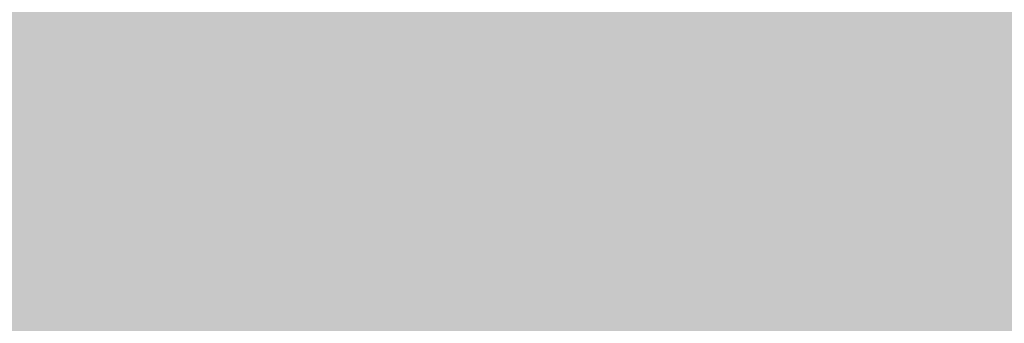
# Model space of a CAD drawing. Units: millimetres. Extents: x 0 to 2267, y 0 to 1823.
# Tile 46 of 256: x 1594.2193 to 1595.0978, y 1226.1145 to 1226.3857. Entities that reach past the tile are written whole.
import ezdxf

# ---------------------------------------------------------------- set-up
doc = ezdxf.new("R2010")
doc.units = ezdxf.units.MM
doc.header["$MEASUREMENT"] = 0
doc.layers.add('M-HATC', color=252, linetype='Continuous', lineweight=18)

msp = doc.modelspace()

# ---------------------------------------------------------------- hatches: boundary and pattern name
at = {"layer": 'M-HATC'}
h = msp.add_hatch(color=256, dxfattribs=at)
h.dxf.hatch_style = 1
h.paths.add_polyline_path([(2055.77105, 1603.06204), (1381.08677, 1603.06204), (1381.08677, 1598.06204), (2055.77105, 1598.06204)])
h.paths.add_polyline_path([(2055.77105, 1598.06204), (1381.08677, 1598.06204), (1381.08677, 1593.06204), (2055.77105, 1593.06204)])
h.paths.add_polyline_path([(2051.30737, 1536.76088), (1385.55044, 1536.76088), (1385.55044, 1526.76088), (1387.55044, 1526.76088), (1388.53662, 1525.05276), (1385.33187, 1521.23348), (1385.33187, 1521.22256), (2050.25417, 1522.74913), (2048.32119, 1525.05276), (2049.30737, 1526.76088), (2051.30737, 1526.76088)])
edge = h.paths.add_edge_path()
edge.add_arc((1847.53451, 1379.14917), 135, 222.6030607, 222.8908505, ccw=False)
edge.add_line((1748.16629, 1287.76561), (1683.09212, 1287.76561))
edge.add_arc((1583.7239, 1379.14917), 135, 317.1091495, 317.3969393, ccw=False)
edge.add_arc((1678.9686, 1290.67067), 5, 222.89085, 317.10915, ccw=False)
edge.add_arc((1774.21331, 1379.14917), 135, 222.6030607, 222.8908505, ccw=False)
edge.add_line((1674.84509, 1287.76561), (1609.77092, 1287.76561))
edge.add_arc((1510.4027, 1379.14917), 135, 317.1091495, 317.3969393, ccw=False)
edge.add_arc((1605.6474, 1290.67067), 5, 222.89085, 317.10915, ccw=False)
edge.add_arc((1700.89211, 1379.14917), 135, 222.6030607, 222.8908505, ccw=False)
edge.add_line((1601.52388, 1287.76561), (1536.44972, 1287.76561))
edge.add_arc((1437.08149, 1379.14917), 135, 317.1091495, 317.3969393, ccw=False)
edge.add_arc((1532.3262, 1290.67067), 5, 222.89085, 317.10915, ccw=False)
edge.add_arc((1627.57091, 1379.14917), 135, 222.6030607, 222.8908505, ccw=False)
edge.add_line((1528.20268, 1287.76561), (1505.92891, 1287.76561))
edge.add_spline(control_points=[(1505.92891, 1287.76561), (1504.26224, 1287.76561), (1504.26224, 1282.76561), (1505.92891, 1282.76561)], knot_values=[0, 0, 0, 0, 5, 5, 5, 5], degree=3, periodic=0)
edge.add_line((1505.92891, 1282.76561), (1930.92891, 1282.76561))
edge.add_spline(control_points=[(1930.92891, 1282.76561), (1932.59557, 1282.76561), (1932.59557, 1287.76561), (1930.92891, 1287.76561)], knot_values=[0, 0, 0, 0, 5, 5, 5, 5], degree=3, periodic=0)
edge.add_line((1930.92891, 1287.76561), (1903.05573, 1287.76561))
edge.add_arc((1803.6875, 1379.14917), 135, 317.1091495, 317.3969393, ccw=False)
edge.add_arc((1898.93221, 1290.67067), 5, 222.89085, 317.10915, ccw=False)
edge.add_arc((1994.17691, 1379.14917), 135, 222.6030607, 222.8908505, ccw=False)
edge.add_line((1894.80869, 1287.76561), (1829.73452, 1287.76561))
edge.add_arc((1730.3663, 1379.14917), 135, 317.1091495, 317.3969393, ccw=False)
edge.add_arc((1825.61101, 1290.67067), 5, 222.89085, 317.10915, ccw=False)
edge.add_arc((1920.85571, 1379.14917), 135, 222.6030607, 222.8908505, ccw=False)
edge.add_line((1821.48749, 1287.76561), (1756.41332, 1287.76561))
edge.add_arc((1657.0451, 1379.14917), 135, 317.1091495, 317.3969393, ccw=False)
edge.add_arc((1752.28981, 1290.67067), 5, 222.89085, 317.10915, ccw=False)
edge = h.paths.add_edge_path()
edge.add_spline(control_points=[(1843.42891, 1227.24746), (1845.09557, 1227.24746), (1845.09557, 1232.24746), (1843.42891, 1232.24746)], knot_values=[0, 0, 0, 0, 5, 5, 5, 5], degree=3, periodic=0)
edge.add_line((1843.42891, 1232.24746), (1593.42891, 1232.24746))
edge.add_spline(control_points=[(1593.42891, 1232.24746), (1591.76224, 1232.24746), (1591.76224, 1227.24746), (1593.42891, 1227.24746)], knot_values=[0, 0, 0, 0, 5, 5, 5, 5], degree=3, periodic=0)
edge.add_line((1593.42891, 1227.24746), (1843.42891, 1227.24746))
h.paths.add_polyline_path([(1905.92891, 1127.41706), (1530.92891, 1127.41706, 0.414214), (1520.92891, 1117.41706), (1530.92891, 1117.41706), (1915.92891, 1117.41706, 0.414214)])
edge = h.paths.add_edge_path()
edge.add_arc((1397.08577, 1498.40775), 12.72993, 90.782146, 190.878706, ccw=False)
edge.add_line((1396.912, 1511.13649), (1428.00968, 1511.34875))
edge.add_line((1428.00968, 1511.34875), (1433.00968, 1511.34875))
edge.add_line((1433.00968, 1511.34875), (1434.439, 1511.34875))
edge.add_arc((1419.474, 1498.08041), 20, 41.560995, 74.082109)
edge.add_line((1424.95919, 1517.31353), (1399.93509, 1517.25608))
edge.add_spline(control_points=[(1399.93074, 1517.25607), (1399.88398, 1517.21312), (1399.8328, 1517.16893), (1399.77741, 1517.1236)], knot_values=[11.567499, 11.567499, 11.567499, 11.567499, 11.814249, 11.814249, 11.814249, 11.814249], degree=3, periodic=0)
edge.add_spline(control_points=[(1399.63279, 1517.00986), (1399.58305, 1516.97214), (1399.53072, 1516.93375), (1399.47591, 1516.89474)], knot_values=[11.167718, 11.167718, 11.167718, 11.167718, 11.365188, 11.365188, 11.365188, 11.365188], degree=3, periodic=0)
edge.add_spline(control_points=[(1399.33981, 1516.80007), (1399.15144, 1516.67185), (1398.93836, 1516.5377), (1398.70404, 1516.39942)], knot_values=[10.376405, 10.376405, 10.376405, 10.376405, 11.00994, 11.00994, 11.00994, 11.00994], degree=3, periodic=0)
edge.add_spline(control_points=[(1398.65716, 1516.37187), (1398.57885, 1516.32602), (1398.49825, 1516.27974), (1398.41549, 1516.23309)], knot_values=[10.125175, 10.125175, 10.125175, 10.125175, 10.334406, 10.334406, 10.334406, 10.334406], degree=3, periodic=0)
edge.add_spline(control_points=[(1398.26422, 1516.14874), (1398.19595, 1516.11107), (1398.12634, 1516.07319), (1398.05546, 1516.03513)], knot_values=[9.832246, 9.832246, 9.832246, 9.832246, 9.999658, 9.999658, 9.999658, 9.999658], degree=3, periodic=0)
edge.add_spline(control_points=[(1397.9987, 1516.00476), (1397.73115, 1515.86211), (1397.44602, 1515.71707), (1397.14664, 1515.57138)], knot_values=[9.161808, 9.161808, 9.161808, 9.161808, 9.787769, 9.787769, 9.787769, 9.787769], degree=3, periodic=0)
edge.add_spline(control_points=[(1397.14664, 1515.57138), (1396.84182, 1515.42305), (1396.52223, 1515.27404), (1396.1914, 1515.12621)], knot_values=[8.524455, 8.524455, 8.524455, 8.524455, 9.161808, 9.161808, 9.161808, 9.161808], degree=3, periodic=0)
edge.add_spline(control_points=[(1396.07771, 1515.07565), (1395.98538, 1515.03478), (1395.89222, 1514.99402), (1395.7983, 1514.9534)], knot_values=[8.275193, 8.275193, 8.275193, 8.275193, 8.451726, 8.451726, 8.451726, 8.451726], degree=3, periodic=0)
edge.add_spline(control_points=[(1395.60184, 1514.86912), (1395.49975, 1514.82568), (1395.39685, 1514.78244), (1395.29322, 1514.73944)], knot_values=[7.962917, 7.962917, 7.962917, 7.962917, 8.152764, 8.152764, 8.152764, 8.152764], degree=3, periodic=0)
edge.add_spline(control_points=[(1395.21158, 1514.70568), (1394.82779, 1514.5475), (1394.43452, 1514.39287), (1394.03645, 1514.24422)], knot_values=[7.21254, 7.21254, 7.21254, 7.21254, 7.913148, 7.913148, 7.913148, 7.913148], degree=3, periodic=0)
edge.add_spline(control_points=[(1394.03645, 1514.24422), (1393.70758, 1514.12142), (1393.37544, 1514.0027), (1393.04267, 1513.88945)], knot_values=[6.633733, 6.633733, 6.633733, 6.633733, 7.21254, 7.21254, 7.21254, 7.21254], degree=3, periodic=0)
edge.add_spline(control_points=[(1392.82142, 1513.81499), (1392.71978, 1513.78118), (1392.61815, 1513.74791), (1392.51658, 1513.71521)], knot_values=[6.328796, 6.328796, 6.328796, 6.328796, 6.505493, 6.505493, 6.505493, 6.505493], degree=3, periodic=0)
edge.add_spline(control_points=[(1392.51658, 1513.71521), (1392.31873, 1513.65151), (1392.12116, 1513.59001), (1391.92441, 1513.53098)], knot_values=[5.984605, 5.984605, 5.984605, 5.984605, 6.328796, 6.328796, 6.328796, 6.328796], degree=3, periodic=0)
edge.add_spline(control_points=[(1391.79155, 1513.49146), (1391.31215, 1513.35011), (1390.83842, 1513.22392), (1390.37844, 1513.11711)], knot_values=[5.066697, 5.066697, 5.066697, 5.066697, 5.907055, 5.907055, 5.907055, 5.907055], degree=3, periodic=0)
edge.add_spline(control_points=[(1390.37844, 1513.11711), (1390.17973, 1513.07097), (1389.98359, 1513.02845), (1389.79067, 1512.98988)], knot_values=[4.70367, 4.70367, 4.70367, 4.70367, 5.066695, 5.066695, 5.066695, 5.066695], degree=3, periodic=0)
edge.add_spline(control_points=[(1389.42203, 1512.92036), (1389.24588, 1512.88922), (1389.0729, 1512.86172), (1388.90364, 1512.83814)], knot_values=[4.130571, 4.130571, 4.130571, 4.130571, 4.469816, 4.469816, 4.469816, 4.469816], degree=3, periodic=0)
edge.add_spline(control_points=[(1388.90364, 1512.83814), (1388.59103, 1512.7946), (1388.29108, 1512.76444), (1388.00714, 1512.74941)], knot_values=[3.504031, 3.504031, 3.504031, 3.504031, 4.130571, 4.130571, 4.130571, 4.130571], degree=3, periodic=0)
edge.add_spline(control_points=[(1387.9356, 1512.74593), (1387.85378, 1512.74231), (1387.77334, 1512.73997), (1387.69435, 1512.73898)], knot_values=[3.268866, 3.268866, 3.268866, 3.268866, 3.451164, 3.451164, 3.451164, 3.451164], degree=3, periodic=0)
edge.add_spline(control_points=[(1387.33512, 1512.74426), (1387.20757, 1512.74991), (1387.08472, 1512.7597), (1386.96699, 1512.77385)], knot_values=[2.670686, 2.670686, 2.670686, 2.670686, 2.984, 2.984, 2.984, 2.984], degree=3, periodic=0)
edge.add_spline(control_points=[(1386.83274, 1512.79225), (1386.82093, 1512.79407), (1386.80917, 1512.79594), (1386.79747, 1512.79787)], knot_values=[2.516981, 2.516981, 2.516981, 2.516981, 2.549528, 2.549528, 2.549528, 2.549528], degree=3, periodic=0)
edge.add_spline(control_points=[(1386.45257, 1512.87348), (1386.42573, 1512.88105), (1386.39931, 1512.88895), (1386.3733, 1512.89719)], knot_values=[2.095869, 2.095869, 2.095869, 2.095869, 2.17941, 2.17941, 2.17941, 2.17941], degree=3, periodic=0)
edge.add_spline(control_points=[(1386.06911, 1513.01889), (1386.06338, 1513.02174), (1386.05768, 1513.02463), (1386.05201, 1513.02753)], knot_values=[1.72453, 1.72453, 1.72453, 1.72453, 1.745933, 1.745933, 1.745933, 1.745933], degree=3, periodic=0)
edge.add_arc((1399.474, 1498.08041), 20, 131.824322, 180)
edge.add_arc((1630.33362, 1505.54843), 250.97076, 181.7051759, 236.427975)
edge.add_arc((1605.33992, 1483.30441), 218.7822, 238.660829, 243.3496099)
edge.add_arc((1647.09105, 1510.35917), 262.89859, 183.1298361, 237.8534422, ccw=False)
h.paths.add_polyline_path([(1406.53685, 1391.96444, 0.149382), (1491.55061, 1296.44177, -0.129517)], flags=17)
edge = h.paths.add_edge_path()
edge.add_arc((2037.38381, 1498.08041), 20, 0, 48.265868)
edge.add_spline(control_points=[(2050.69731, 1513.00525), (2050.65121, 1512.98471), (2050.60338, 1512.96554), (2050.55388, 1512.94771)], knot_values=[1.835652, 1.835652, 1.835652, 1.835652, 2.000781, 2.000781, 2.000781, 2.000781], degree=3, periodic=0)
edge.add_spline(control_points=[(2050.46156, 1512.91661), (2050.479, 1512.9221), (2050.49625, 1512.92774), (2050.51332, 1512.93353)], knot_values=[2.045477, 2.045477, 2.045477, 2.045477, 2.101389, 2.101389, 2.101389, 2.101389], degree=3, periodic=0)
edge.add_spline(control_points=[(2050.12896, 1512.83416), (2050.19843, 1512.84734), (2050.26573, 1512.86233), (2050.33075, 1512.87919)], knot_values=[2.237629, 2.237629, 2.237629, 2.237629, 2.435841, 2.435841, 2.435841, 2.435841], degree=3, periodic=0)
edge.add_spline(control_points=[(2050.09463, 1512.82783), (2050.10613, 1512.82989), (2050.11757, 1512.832), (2050.12896, 1512.83416)], knot_values=[2.435841, 2.435841, 2.435841, 2.435841, 2.468321, 2.468321, 2.468321, 2.468321], degree=3, periodic=0)
edge.add_spline(control_points=[(2049.78433, 1512.78511), (2049.85521, 1512.79219), (2049.92435, 1512.80077), (2049.99166, 1512.81088)], knot_values=[2.563852, 2.563852, 2.563852, 2.563852, 2.748541, 2.748541, 2.748541, 2.748541], degree=3, periodic=0)
edge.add_spline(control_points=[(2049.4052, 1512.76169), (2049.5364, 1512.76526), (2049.66292, 1512.77299), (2049.78433, 1512.78511)], knot_values=[2.748541, 2.748541, 2.748541, 2.748541, 3.064882, 3.064882, 3.064882, 3.064882], degree=3, periodic=0)
edge.add_spline(control_points=[(2049.16976, 1512.75968), (2049.23364, 1512.7591), (2049.29654, 1512.7594), (2049.35844, 1512.7606)], knot_values=[3.102309, 3.102309, 3.102309, 3.102309, 3.2503, 3.2503, 3.2503, 3.2503], degree=3, periodic=0)
edge.add_spline(control_points=[(2048.85727, 1512.76911), (2048.96378, 1512.76378), (2049.068, 1512.76061), (2049.16976, 1512.75968)], knot_values=[3.2503, 3.2503, 3.2503, 3.2503, 3.486069, 3.486069, 3.486069, 3.486069], degree=3, periodic=0)
edge.add_spline(control_points=[(2048.69241, 1512.77892), (2048.3729, 1512.80093), (2048.0345, 1512.84106), (2047.68175, 1512.89697)], knot_values=[3.606429, 3.606429, 3.606429, 3.606429, 4.2989, 4.2989, 4.2989, 4.2989], degree=3, periodic=0)
edge.add_spline(control_points=[(2047.68175, 1512.89697), (2047.5458, 1512.91852), (2047.40772, 1512.94241), (2047.26776, 1512.96851)], knot_values=[4.2989, 4.2989, 4.2989, 4.2989, 4.565769, 4.565769, 4.565769, 4.565769], degree=3, periodic=0)
edge.add_spline(control_points=[(2047.26776, 1512.96851), (2047.14494, 1512.99141), (2047.02067, 1513.01601), (2046.89514, 1513.04223)], knot_values=[4.565769, 4.565769, 4.565769, 4.565769, 4.799971, 4.799971, 4.799971, 4.799971], degree=3, periodic=0)
edge.add_spline(control_points=[(2046.89514, 1513.04223), (2046.52865, 1513.11875), (2046.15135, 1513.20899), (2045.7676, 1513.31068)], knot_values=[4.799971, 4.799971, 4.799971, 4.799971, 5.483718, 5.483718, 5.483718, 5.483718], degree=3, periodic=0)
edge.add_spline(control_points=[(2045.7676, 1513.31068), (2045.3724, 1513.41539), (2044.97036, 1513.53225), (2044.56625, 1513.65876)], knot_values=[5.483718, 5.483718, 5.483718, 5.483718, 6.187866, 6.187866, 6.187866, 6.187866], degree=3, periodic=0)
edge.add_spline(control_points=[(2044.56625, 1513.65876), (2044.41491, 1513.70614), (2044.26329, 1513.75487), (2044.11163, 1513.80482)], knot_values=[6.187866, 6.187866, 6.187866, 6.187866, 6.451551, 6.451551, 6.451551, 6.451551], degree=3, periodic=0)
edge.add_spline(control_points=[(2044.11163, 1513.80482), (2043.99666, 1513.84269), (2043.88167, 1513.88126), (2043.76676, 1513.92048)], knot_values=[6.451551, 6.451551, 6.451551, 6.451551, 6.651434, 6.651434, 6.651434, 6.651434], degree=3, periodic=0)
edge.add_spline(control_points=[(2043.76676, 1513.92048), (2043.37157, 1514.05536), (2042.97738, 1514.19789), (2042.58863, 1514.34575)], knot_values=[6.651434, 6.651434, 6.651434, 6.651434, 7.338879, 7.338879, 7.338879, 7.338879], degree=3, periodic=0)
edge.add_spline(control_points=[(2042.58863, 1514.34575), (2042.16431, 1514.50715), (2041.74647, 1514.67491), (2041.34086, 1514.84603)], knot_values=[7.338879, 7.338879, 7.338879, 7.338879, 8.089209, 8.089209, 8.089209, 8.089209], degree=3, periodic=0)
edge.add_spline(control_points=[(2041.34086, 1514.84603), (2041.1028, 1514.94647), (2040.86896, 1515.04806), (2040.64049, 1515.1502)], knot_values=[8.089209, 8.089209, 8.089209, 8.089209, 8.529587, 8.529587, 8.529587, 8.529587], degree=3, periodic=0)
edge.add_spline(control_points=[(2040.50999, 1515.20887), (2040.08238, 1515.40218), (2039.67475, 1515.59705), (2039.29495, 1515.78939)], knot_values=[8.613818, 8.613818, 8.613818, 8.613818, 9.44571, 9.44571, 9.44571, 9.44571], degree=3, periodic=0)
edge.add_spline(control_points=[(2039.29495, 1515.78939), (2039.0618, 1515.90746), (2038.83914, 1516.02458), (2038.62878, 1516.1398)], knot_values=[9.44571, 9.44571, 9.44571, 9.44571, 9.956404, 9.956404, 9.956404, 9.956404], degree=3, periodic=0)
edge.add_spline(control_points=[(2038.62878, 1516.1398), (2038.51874, 1516.20007), (2038.41207, 1516.25982), (2038.30903, 1516.31891)], knot_values=[9.956404, 9.956404, 9.956404, 9.956404, 10.223542, 10.223542, 10.223542, 10.223542], degree=3, periodic=0)
edge.add_spline(control_points=[(2038.30903, 1516.31891), (2038.21377, 1516.37354), (2038.12161, 1516.42762), (2038.03275, 1516.48102)], knot_values=[10.223542, 10.223542, 10.223542, 10.223542, 10.47051, 10.47051, 10.47051, 10.47051], degree=3, periodic=0)
edge.add_spline(control_points=[(2038.03275, 1516.48102), (2037.78552, 1516.62961), (2037.56388, 1516.77304), (2037.37225, 1516.909)], knot_values=[10.47051, 10.47051, 10.47051, 10.47051, 11.15767, 11.15767, 11.15767, 11.15767], degree=3, periodic=0)
edge.add_spline(control_points=[(2037.37225, 1516.909), (2037.27893, 1516.9752), (2037.19274, 1517.03963), (2037.11417, 1517.10203)], knot_values=[11.15767, 11.15767, 11.15767, 11.15767, 11.49227, 11.49227, 11.49227, 11.49227], degree=3, periodic=0)
edge.add_spline(control_points=[(2036.85638, 1517.32585), (2036.91481, 1517.26923), (2036.98143, 1517.21027), (2037.05573, 1517.14922)], knot_values=[11.577341, 11.577341, 11.577341, 11.577341, 11.91035, 11.91035, 11.91035, 11.91035], degree=3, periodic=0)
edge.add_spline(control_points=[(2036.80739, 1517.37475), (2036.82301, 1517.35865), (2036.83935, 1517.34235), (2036.85638, 1517.32585)], knot_values=[11.91035, 11.91035, 11.91035, 11.91035, 12.007402, 12.007402, 12.007402, 12.007402], degree=3, periodic=0)
edge.add_spline(control_points=[(2036.70167, 1517.494), (2036.71042, 1517.48299), (2036.71958, 1517.47185), (2036.72913, 1517.4606)], knot_values=[12.184155, 12.184155, 12.184155, 12.184155, 12.255409, 12.255409, 12.255409, 12.255409], degree=3, periodic=0)
edge.add_spline(control_points=[(2036.6159, 1517.6205), (2036.61998, 1517.61304), (2036.6243, 1517.6055), (2036.62885, 1517.59789)], knot_values=[12.487913, 12.487913, 12.487913, 12.487913, 12.541035, 12.541035, 12.541035, 12.541035], degree=3, periodic=0)
edge.add_spline(control_points=[(2036.56349, 1517.78599), (2036.56372, 1517.77936), (2036.56423, 1517.77264), (2036.56502, 1517.76582)], knot_values=[12.911761, 12.911761, 12.911761, 12.911761, 12.968286, 12.968286, 12.968286, 12.968286], degree=3, periodic=0)
edge.add_spline(control_points=[(2036.61663, 1517.93042), (2036.61248, 1517.92586), (2036.60857, 1517.92121), (2036.60491, 1517.91648)], knot_values=[13.382527, 13.382527, 13.382527, 13.382527, 13.433791, 13.433791, 13.433791, 13.433791], degree=3, periodic=0)
edge.add_spline(control_points=[(2036.74902, 1518.01695), (2036.73613, 1518.0116), (2036.72393, 1518.00601), (2036.71242, 1518.00018)], knot_values=[13.726299, 13.726299, 13.726299, 13.726299, 13.809928, 13.809928, 13.809928, 13.809928], degree=3, periodic=0)
edge.add_spline(control_points=[(2036.86043, 1518.05285), (2036.83863, 1518.04743), (2036.81809, 1518.04156), (2036.79879, 1518.03526)], knot_values=[13.910887, 13.910887, 13.910887, 13.910887, 14.02153, 14.02153, 14.02153, 14.02153], degree=3, periodic=0)
edge.add_line((2036.96387, 1518.08041), (2032.38381, 1518.08041))
edge.add_line((2032.38381, 1518.08041), (2027.38381, 1518.08041))
edge.add_line((2027.38381, 1518.08041), (2022.38381, 1518.08041))
edge.add_line((2022.38381, 1518.08041), (2017.38381, 1518.08041))
edge.add_arc((2017.38381, 1498.08041), 20, 90, 138.439005)
edge.add_line((2002.41881, 1511.34875), (2003.84813, 1511.34875))
edge.add_line((2003.84813, 1511.34875), (2008.84813, 1511.34875))
edge.add_line((2008.84813, 1511.34875), (2039.77204, 1511.13768))
edge.add_arc((2039.77204, 1498.40775), 12.72993, -10.878706, 90, ccw=False)
edge.add_arc((1789.76676, 1510.35917), 262.89859, 302.1465578, 356.8701639, ccw=False)
edge.add_arc((1831.51789, 1483.30441), 218.7822, 296.6503901, 301.339171)
edge.add_arc((1806.52419, 1505.54843), 250.97076, 303.572025, 358.2948241)
h.paths.add_polyline_path([(2030.32096, 1391.96444, -0.129517), (1945.3072, 1296.44177, 0.149382)], flags=17)
edge = h.paths.add_edge_path()
edge.add_spline(control_points=[(2037.2464, 1518.08209), (2037.28977, 1518.08098), (2037.33555, 1518.08041), (2037.3838, 1518.08041)], knot_values=[0.000012, 0.000012, 0.000012, 0.000012, 0.144754, 0.144754, 0.144754, 0.144754], degree=3, periodic=0)
edge.add_line((2037.33571, 1518.08041), (2037.00963, 1518.08041))
edge.add_spline(control_points=[(2037.00963, 1518.08041), (2036.98217, 1518.07678), (2036.95605, 1518.07266), (2036.93124, 1518.06808)], knot_values=[14.13465, 14.13465, 14.13465, 14.13465, 14.247197, 14.247197, 14.247197, 14.247197], degree=3, periodic=0)
edge.add_spline(control_points=[(2036.93124, 1518.06808), (2036.92764, 1518.06741), (2036.92407, 1518.06674), (2036.92053, 1518.06605)], knot_values=[14.118315, 14.118315, 14.118315, 14.118315, 14.13465, 14.13465, 14.13465, 14.13465], degree=3, periodic=0)
edge.add_spline(control_points=[(2036.92053, 1518.06605), (2036.9118, 1518.06436), (2036.90323, 1518.06262), (2036.89484, 1518.06081)], knot_values=[14.078086, 14.078086, 14.078086, 14.078086, 14.118315, 14.118315, 14.118315, 14.118315], degree=3, periodic=0)
edge.add_spline(control_points=[(2036.89484, 1518.06081), (2036.88304, 1518.05827), (2036.87157, 1518.05562), (2036.86043, 1518.05285)], knot_values=[14.02153, 14.02153, 14.02153, 14.02153, 14.078086, 14.078086, 14.078086, 14.078086], degree=3, periodic=0)
edge.add_spline(control_points=[(2036.86043, 1518.05285), (2036.83863, 1518.04743), (2036.81809, 1518.04156), (2036.79879, 1518.03526)], knot_values=[13.910887, 13.910887, 13.910887, 13.910887, 14.02153, 14.02153, 14.02153, 14.02153], degree=3, periodic=0)
edge.add_spline(control_points=[(2036.79879, 1518.03526), (2036.79809, 1518.03504), (2036.7974, 1518.03481), (2036.79671, 1518.03458)], knot_values=[13.906906, 13.906906, 13.906906, 13.906906, 13.910887, 13.910887, 13.910887, 13.910887], degree=3, periodic=0)
edge.add_spline(control_points=[(2036.79671, 1518.03458), (2036.78819, 1518.03178), (2036.77991, 1518.02888), (2036.77187, 1518.02591)], knot_values=[13.857826, 13.857826, 13.857826, 13.857826, 13.906906, 13.906906, 13.906906, 13.906906], degree=3, periodic=0)
edge.add_spline(control_points=[(2036.77187, 1518.02591), (2036.76402, 1518.023), (2036.75641, 1518.02002), (2036.74902, 1518.01695)], knot_values=[13.809928, 13.809928, 13.809928, 13.809928, 13.857826, 13.857826, 13.857826, 13.857826], degree=3, periodic=0)
edge.add_spline(control_points=[(2036.74902, 1518.01695), (2036.73613, 1518.0116), (2036.72393, 1518.00601), (2036.71242, 1518.00018)], knot_values=[13.726299, 13.726299, 13.726299, 13.726299, 13.809928, 13.809928, 13.809928, 13.809928], degree=3, periodic=0)
edge.add_spline(control_points=[(2036.71242, 1518.00018), (2036.71211, 1518.00002), (2036.71179, 1517.99986), (2036.71147, 1517.99969)], knot_values=[13.723993, 13.723993, 13.723993, 13.723993, 13.726299, 13.726299, 13.726299, 13.726299], degree=3, periodic=0)
edge.add_spline(control_points=[(2036.71147, 1517.99969), (2036.70634, 1517.99708), (2036.70134, 1517.99441), (2036.69648, 1517.9917)], knot_values=[13.686536, 13.686536, 13.686536, 13.686536, 13.723993, 13.723993, 13.723993, 13.723993], degree=3, periodic=0)
edge.add_spline(control_points=[(2036.69648, 1517.9917), (2036.6919, 1517.98914), (2036.68744, 1517.98654), (2036.6831, 1517.9839)], knot_values=[13.651251, 13.651251, 13.651251, 13.651251, 13.686536, 13.686536, 13.686536, 13.686536], degree=3, periodic=0)
edge.add_spline(control_points=[(2036.6831, 1517.9839), (2036.67641, 1517.97983), (2036.67001, 1517.97566), (2036.6639, 1517.97139)], knot_values=[13.596804, 13.596804, 13.596804, 13.596804, 13.651251, 13.651251, 13.651251, 13.651251], degree=3, periodic=0)
edge.add_spline(control_points=[(2036.6639, 1517.97139), (2036.66358, 1517.97117), (2036.66326, 1517.97094), (2036.66294, 1517.97072)], knot_values=[13.593956, 13.593956, 13.593956, 13.593956, 13.596804, 13.596804, 13.596804, 13.596804], degree=3, periodic=0)
edge.add_spline(control_points=[(2036.66294, 1517.97072), (2036.6603, 1517.96886), (2036.65771, 1517.96698), (2036.65518, 1517.96509)], knot_values=[13.570322, 13.570322, 13.570322, 13.570322, 13.593956, 13.593956, 13.593956, 13.593956], degree=3, periodic=0)
edge.add_spline(control_points=[(2036.65518, 1517.96509), (2036.65251, 1517.9631), (2036.64991, 1517.96108), (2036.64737, 1517.95905)], knot_values=[13.545477, 13.545477, 13.545477, 13.545477, 13.570322, 13.570322, 13.570322, 13.570322], degree=3, periodic=0)
edge.add_spline(control_points=[(2036.64737, 1517.95905), (2036.64721, 1517.95892), (2036.64705, 1517.9588), (2036.64689, 1517.95867)], knot_values=[13.543931, 13.543931, 13.543931, 13.543931, 13.545477, 13.545477, 13.545477, 13.545477], degree=3, periodic=0)
edge.add_spline(control_points=[(2036.64689, 1517.95867), (2036.64121, 1517.95411), (2036.63582, 1517.94945), (2036.63073, 1517.94468)], knot_values=[13.488237, 13.488237, 13.488237, 13.488237, 13.543931, 13.543931, 13.543931, 13.543931], degree=3, periodic=0)
edge.add_spline(control_points=[(2036.63073, 1517.94468), (2036.62817, 1517.94229), (2036.62569, 1517.93988), (2036.62329, 1517.93744)], knot_values=[13.460307, 13.460307, 13.460307, 13.460307, 13.488237, 13.488237, 13.488237, 13.488237], degree=3, periodic=0)
edge.add_spline(control_points=[(2036.62329, 1517.93744), (2036.62151, 1517.93564), (2036.61978, 1517.93383), (2036.61809, 1517.932)], knot_values=[13.439712, 13.439712, 13.439712, 13.439712, 13.460307, 13.460307, 13.460307, 13.460307], degree=3, periodic=0)
edge.add_spline(control_points=[(2036.61809, 1517.932), (2036.6176, 1517.93147), (2036.61711, 1517.93095), (2036.61663, 1517.93042)], knot_values=[13.433791, 13.433791, 13.433791, 13.433791, 13.439712, 13.439712, 13.439712, 13.439712], degree=3, periodic=0)
edge.add_spline(control_points=[(2036.61663, 1517.93042), (2036.61248, 1517.92586), (2036.60857, 1517.92121), (2036.60491, 1517.91648)], knot_values=[13.382527, 13.382527, 13.382527, 13.382527, 13.433791, 13.433791, 13.433791, 13.433791], degree=3, periodic=0)
edge.add_spline(control_points=[(2036.60491, 1517.91648), (2036.60258, 1517.91347), (2036.60036, 1517.91044), (2036.59824, 1517.90737)], knot_values=[13.350017, 13.350017, 13.350017, 13.350017, 13.382527, 13.382527, 13.382527, 13.382527], degree=3, periodic=0)
edge.add_spline(control_points=[(2036.59824, 1517.90737), (2036.59718, 1517.90585), (2036.59616, 1517.90433), (2036.59515, 1517.90279)], knot_values=[13.333922, 13.333922, 13.333922, 13.333922, 13.350017, 13.350017, 13.350017, 13.350017], degree=3, periodic=0)
edge.add_spline(control_points=[(2036.59515, 1517.90279), (2036.59452, 1517.90183), (2036.5939, 1517.90086), (2036.59329, 1517.89989)], knot_values=[13.323828, 13.323828, 13.323828, 13.323828, 13.333922, 13.333922, 13.333922, 13.333922], degree=3, periodic=0)
edge.add_spline(control_points=[(2036.59329, 1517.89989), (2036.59049, 1517.89545), (2036.5879, 1517.89094), (2036.5855, 1517.88637)], knot_values=[13.277545, 13.277545, 13.277545, 13.277545, 13.323828, 13.323828, 13.323828, 13.323828], degree=3, periodic=0)
edge.add_spline(control_points=[(2036.5855, 1517.88637), (2036.58355, 1517.88267), (2036.58174, 1517.87892), (2036.58006, 1517.87513)], knot_values=[13.240119, 13.240119, 13.240119, 13.240119, 13.277545, 13.277545, 13.277545, 13.277545], degree=3, periodic=0)
edge.add_spline(control_points=[(2036.58006, 1517.87513), (2036.57952, 1517.87393), (2036.579, 1517.87272), (2036.57849, 1517.87151)], knot_values=[13.228211, 13.228211, 13.228211, 13.228211, 13.240119, 13.240119, 13.240119, 13.240119], degree=3, periodic=0)
edge.add_spline(control_points=[(2036.57849, 1517.87151), (2036.57796, 1517.87023), (2036.57744, 1517.86896), (2036.57693, 1517.86767)], knot_values=[13.215717, 13.215717, 13.215717, 13.215717, 13.228211, 13.228211, 13.228211, 13.228211], degree=3, periodic=0)
edge.add_spline(control_points=[(2036.57693, 1517.86767), (2036.57548, 1517.86399), (2036.57414, 1517.86027), (2036.57293, 1517.85651)], knot_values=[13.179847, 13.179847, 13.179847, 13.179847, 13.215717, 13.215717, 13.215717, 13.215717], degree=3, periodic=0)
edge.add_spline(control_points=[(2036.57293, 1517.85651), (2036.5713, 1517.8515), (2036.56989, 1517.84641), (2036.56868, 1517.84126)], knot_values=[13.132017, 13.132017, 13.132017, 13.132017, 13.179847, 13.179847, 13.179847, 13.179847], degree=3, periodic=0)
edge.add_spline(control_points=[(2036.56868, 1517.84126), (2036.56844, 1517.84023), (2036.56821, 1517.8392), (2036.56798, 1517.83817)], knot_values=[13.122482, 13.122482, 13.122482, 13.122482, 13.132017, 13.132017, 13.132017, 13.132017], degree=3, periodic=0)
edge.add_spline(control_points=[(2036.56798, 1517.83817), (2036.56758, 1517.83634), (2036.56721, 1517.8345), (2036.56687, 1517.83266)], knot_values=[13.105592, 13.105592, 13.105592, 13.105592, 13.122482, 13.122482, 13.122482, 13.122482], degree=3, periodic=0)
edge.add_spline(control_points=[(2036.56687, 1517.83266), (2036.56622, 1517.82921), (2036.56567, 1517.82574), (2036.5652, 1517.82223)], knot_values=[13.074063, 13.074063, 13.074063, 13.074063, 13.105592, 13.105592, 13.105592, 13.105592], degree=3, periodic=0)
edge.add_spline(control_points=[(2036.5652, 1517.82223), (2036.5652, 1517.82223), (2036.5652, 1517.82223), (2036.5652, 1517.82223)], knot_values=[13.074043, 13.074043, 13.074043, 13.074043, 13.074063, 13.074063, 13.074063, 13.074063], degree=3, periodic=0)
edge.add_spline(control_points=[(2036.5652, 1517.82223), (2036.56443, 1517.81643), (2036.5639, 1517.81055), (2036.56361, 1517.8046)], knot_values=[13.021884, 13.021884, 13.021884, 13.021884, 13.074043, 13.074043, 13.074043, 13.074043], degree=3, periodic=0)
edge.add_spline(control_points=[(2036.56361, 1517.8046), (2036.56358, 1517.80401), (2036.56356, 1517.80342), (2036.56353, 1517.80283)], knot_values=[13.01674, 13.01674, 13.01674, 13.01674, 13.021884, 13.021884, 13.021884, 13.021884], degree=3, periodic=0)
edge.add_spline(control_points=[(2036.56353, 1517.80283), (2036.56344, 1517.80051), (2036.56338, 1517.79817), (2036.56336, 1517.79582)], knot_values=[12.996438, 12.996438, 12.996438, 12.996438, 13.01674, 13.01674, 13.01674, 13.01674], degree=3, periodic=0)
edge.add_spline(control_points=[(2036.56336, 1517.79582), (2036.56334, 1517.79257), (2036.56338, 1517.78929), (2036.56349, 1517.78599)], knot_values=[12.968286, 12.968286, 12.968286, 12.968286, 12.996438, 12.996438, 12.996438, 12.996438], degree=3, periodic=0)
edge.add_spline(control_points=[(2036.56349, 1517.78599), (2036.56372, 1517.77936), (2036.56423, 1517.77264), (2036.56502, 1517.76582)], knot_values=[12.911761, 12.911761, 12.911761, 12.911761, 12.968286, 12.968286, 12.968286, 12.968286], degree=3, periodic=0)
edge.add_spline(control_points=[(2036.56502, 1517.76582), (2036.56503, 1517.76573), (2036.56504, 1517.76564), (2036.56505, 1517.76555)], knot_values=[12.911017, 12.911017, 12.911017, 12.911017, 12.911761, 12.911761, 12.911761, 12.911761], degree=3, periodic=0)
edge.add_spline(control_points=[(2036.56505, 1517.76555), (2036.56541, 1517.76245), (2036.56583, 1517.75933), (2036.56631, 1517.75619)], knot_values=[12.88528, 12.88528, 12.88528, 12.88528, 12.911017, 12.911017, 12.911017, 12.911017], degree=3, periodic=0)
edge.add_spline(control_points=[(2036.56631, 1517.75619), (2036.56673, 1517.75341), (2036.5672, 1517.75062), (2036.56771, 1517.74782)], knot_values=[12.862519, 12.862519, 12.862519, 12.862519, 12.88528, 12.88528, 12.88528, 12.88528], degree=3, periodic=0)
edge.add_spline(control_points=[(2036.56771, 1517.74782), (2036.56779, 1517.74737), (2036.56788, 1517.74692), (2036.56796, 1517.74647)], knot_values=[12.858885, 12.858885, 12.858885, 12.858885, 12.862519, 12.862519, 12.862519, 12.862519], degree=3, periodic=0)
edge.add_spline(control_points=[(2036.56796, 1517.74647), (2036.5692, 1517.73986), (2036.57069, 1517.73316), (2036.57243, 1517.72638)], knot_values=[12.8053, 12.8053, 12.8053, 12.8053, 12.858885, 12.858885, 12.858885, 12.858885], degree=3, periodic=0)
edge.add_spline(control_points=[(2036.57243, 1517.72638), (2036.5734, 1517.72257), (2036.57446, 1517.71874), (2036.57559, 1517.71488)], knot_values=[12.775176, 12.775176, 12.775176, 12.775176, 12.8053, 12.8053, 12.8053, 12.8053], degree=3, periodic=0)
edge.add_spline(control_points=[(2036.57559, 1517.71488), (2036.57628, 1517.71252), (2036.577, 1517.71015), (2036.57775, 1517.70778)], knot_values=[12.756759, 12.756759, 12.756759, 12.756759, 12.775176, 12.775176, 12.775176, 12.775176], degree=3, periodic=0)
edge.add_spline(control_points=[(2036.57775, 1517.70778), (2036.57808, 1517.70674), (2036.57841, 1517.7057), (2036.57875, 1517.70466)], knot_values=[12.748742, 12.748742, 12.748742, 12.748742, 12.756759, 12.756759, 12.756759, 12.756759], degree=3, periodic=0)
edge.add_spline(control_points=[(2036.57875, 1517.70466), (2036.58082, 1517.6983), (2036.58309, 1517.69187), (2036.58557, 1517.68537)], knot_values=[12.69959, 12.69959, 12.69959, 12.69959, 12.748742, 12.748742, 12.748742, 12.748742], degree=3, periodic=0)
edge.add_spline(control_points=[(2036.58557, 1517.68537), (2036.58762, 1517.68001), (2036.5898, 1517.6746), (2036.59213, 1517.66916)], knot_values=[12.659038, 12.659038, 12.659038, 12.659038, 12.69959, 12.69959, 12.69959, 12.69959], degree=3, periodic=0)
edge.add_spline(control_points=[(2036.59213, 1517.66916), (2036.59397, 1517.66482), (2036.59591, 1517.66047), (2036.59793, 1517.65608)], knot_values=[12.626806, 12.626806, 12.626806, 12.626806, 12.659038, 12.659038, 12.659038, 12.659038], degree=3, periodic=0)
edge.add_spline(control_points=[(2036.59793, 1517.65608), (2036.59839, 1517.65507), (2036.59886, 1517.65406), (2036.59934, 1517.65305)], knot_values=[12.619394, 12.619394, 12.619394, 12.619394, 12.626806, 12.626806, 12.626806, 12.626806], degree=3, periodic=0)
edge.add_spline(control_points=[(2036.59934, 1517.65305), (2036.60435, 1517.64236), (2036.60987, 1517.63151), (2036.61589, 1517.6205)], knot_values=[12.541039, 12.541039, 12.541039, 12.541039, 12.619394, 12.619394, 12.619394, 12.619394], degree=3, periodic=0)
edge.add_spline(control_points=[(2036.61589, 1517.6205), (2036.61589, 1517.6205), (2036.6159, 1517.6205), (2036.6159, 1517.6205)], knot_values=[12.541035, 12.541035, 12.541035, 12.541035, 12.541039, 12.541039, 12.541039, 12.541039], degree=3, periodic=0)
edge.add_spline(control_points=[(2036.6159, 1517.6205), (2036.61998, 1517.61304), (2036.6243, 1517.6055), (2036.62885, 1517.59789)], knot_values=[12.487913, 12.487913, 12.487913, 12.487913, 12.541035, 12.541035, 12.541035, 12.541035], degree=3, periodic=0)
edge.add_spline(control_points=[(2036.62885, 1517.59789), (2036.63261, 1517.5916), (2036.63653, 1517.58526), (2036.64061, 1517.57888)], knot_values=[12.443982, 12.443982, 12.443982, 12.443982, 12.487913, 12.487913, 12.487913, 12.487913], degree=3, periodic=0)
edge.add_spline(control_points=[(2036.64061, 1517.57888), (2036.64144, 1517.57757), (2036.64228, 1517.57626), (2036.64313, 1517.57495)], knot_values=[12.434996, 12.434996, 12.434996, 12.434996, 12.443982, 12.443982, 12.443982, 12.443982], degree=3, periodic=0)
edge.add_spline(control_points=[(2036.64313, 1517.57495), (2036.65306, 1517.55958), (2036.66389, 1517.54394), (2036.6756, 1517.52803)], knot_values=[12.329647, 12.329647, 12.329647, 12.329647, 12.434996, 12.434996, 12.434996, 12.434996], degree=3, periodic=0)
edge.add_spline(control_points=[(2036.6756, 1517.52803), (2036.68385, 1517.51682), (2036.69254, 1517.50548), (2036.70167, 1517.494)], knot_values=[12.255409, 12.255409, 12.255409, 12.255409, 12.329647, 12.329647, 12.329647, 12.329647], degree=3, periodic=0)
edge.add_spline(control_points=[(2036.70167, 1517.494), (2036.71042, 1517.48299), (2036.71958, 1517.47185), (2036.72913, 1517.4606)], knot_values=[12.184155, 12.184155, 12.184155, 12.184155, 12.255409, 12.255409, 12.255409, 12.255409], degree=3, periodic=0)
edge.add_spline(control_points=[(2036.72913, 1517.4606), (2036.74363, 1517.44352), (2036.75904, 1517.42617), (2036.77534, 1517.40855)], knot_values=[12.075961, 12.075961, 12.075961, 12.075961, 12.184155, 12.184155, 12.184155, 12.184155], degree=3, periodic=0)
edge.add_spline(control_points=[(2036.77534, 1517.40855), (2036.77631, 1517.4075), (2036.77729, 1517.40645), (2036.77827, 1517.40539)], knot_values=[12.069502, 12.069502, 12.069502, 12.069502, 12.075961, 12.075961, 12.075961, 12.075961], degree=3, periodic=0)
edge.add_spline(control_points=[(2036.77827, 1517.40539), (2036.78768, 1517.39526), (2036.79739, 1517.38505), (2036.80739, 1517.37475)], knot_values=[12.007402, 12.007402, 12.007402, 12.007402, 12.069502, 12.069502, 12.069502, 12.069502], degree=3, periodic=0)
edge.add_spline(control_points=[(2036.80739, 1517.37475), (2036.82301, 1517.35865), (2036.83935, 1517.34235), (2036.85638, 1517.32585)], knot_values=[11.91035, 11.91035, 11.91035, 11.91035, 12.007402, 12.007402, 12.007402, 12.007402], degree=3, periodic=0)
edge.add_spline(control_points=[(2036.85638, 1517.32585), (2036.91481, 1517.26923), (2036.98143, 1517.21027), (2037.05573, 1517.14922)], knot_values=[11.577341, 11.577341, 11.577341, 11.577341, 11.91035, 11.91035, 11.91035, 11.91035], degree=3, periodic=0)
edge.add_spline(control_points=[(2037.05573, 1517.14922), (2037.07471, 1517.13362), (2037.0942, 1517.11789), (2037.11417, 1517.10203)], knot_values=[11.49227, 11.49227, 11.49227, 11.49227, 11.577341, 11.577341, 11.577341, 11.577341], degree=3, periodic=0)
edge.add_spline(control_points=[(2037.11417, 1517.10203), (2037.19274, 1517.03963), (2037.27893, 1516.9752), (2037.37225, 1516.909)], knot_values=[11.15767, 11.15767, 11.15767, 11.15767, 11.49227, 11.49227, 11.49227, 11.49227], degree=3, periodic=0)
edge.add_spline(control_points=[(2037.37225, 1516.909), (2037.56388, 1516.77304), (2037.78552, 1516.62961), (2038.03275, 1516.48102)], knot_values=[10.47051, 10.47051, 10.47051, 10.47051, 11.15767, 11.15767, 11.15767, 11.15767], degree=3, periodic=0)
edge.add_spline(control_points=[(2038.03275, 1516.48102), (2038.12161, 1516.42762), (2038.21377, 1516.37354), (2038.30903, 1516.31891)], knot_values=[10.223542, 10.223542, 10.223542, 10.223542, 10.47051, 10.47051, 10.47051, 10.47051], degree=3, periodic=0)
edge.add_spline(control_points=[(2038.30903, 1516.31891), (2038.41207, 1516.25982), (2038.51874, 1516.20007), (2038.62878, 1516.1398)], knot_values=[9.956404, 9.956404, 9.956404, 9.956404, 10.223542, 10.223542, 10.223542, 10.223542], degree=3, periodic=0)
edge.add_spline(control_points=[(2038.62878, 1516.1398), (2038.83914, 1516.02458), (2039.0618, 1515.90746), (2039.29495, 1515.78939)], knot_values=[9.44571, 9.44571, 9.44571, 9.44571, 9.956404, 9.956404, 9.956404, 9.956404], degree=3, periodic=0)
edge.add_spline(control_points=[(2039.29495, 1515.78939), (2039.67475, 1515.59705), (2040.08238, 1515.40218), (2040.50999, 1515.20887)], knot_values=[8.613818, 8.613818, 8.613818, 8.613818, 9.44571, 9.44571, 9.44571, 9.44571], degree=3, periodic=0)
edge.add_spline(control_points=[(2040.50999, 1515.20887), (2040.55329, 1515.1893), (2040.59679, 1515.16974), (2040.64049, 1515.1502)], knot_values=[8.529587, 8.529587, 8.529587, 8.529587, 8.613818, 8.613818, 8.613818, 8.613818], degree=3, periodic=0)
edge.add_spline(control_points=[(2040.64049, 1515.1502), (2040.86896, 1515.04806), (2041.1028, 1514.94647), (2041.34086, 1514.84603)], knot_values=[8.089209, 8.089209, 8.089209, 8.089209, 8.529587, 8.529587, 8.529587, 8.529587], degree=3, periodic=0)
edge.add_spline(control_points=[(2041.34086, 1514.84603), (2041.74647, 1514.67491), (2042.16431, 1514.50715), (2042.58863, 1514.34575)], knot_values=[7.338879, 7.338879, 7.338879, 7.338879, 8.089209, 8.089209, 8.089209, 8.089209], degree=3, periodic=0)
edge.add_spline(control_points=[(2042.58863, 1514.34575), (2042.97738, 1514.19789), (2043.37157, 1514.05536), (2043.76676, 1513.92048)], knot_values=[6.651434, 6.651434, 6.651434, 6.651434, 7.338879, 7.338879, 7.338879, 7.338879], degree=3, periodic=0)
edge.add_spline(control_points=[(2043.76676, 1513.92048), (2043.88167, 1513.88126), (2043.99666, 1513.84269), (2044.11163, 1513.80482)], knot_values=[6.451551, 6.451551, 6.451551, 6.451551, 6.651434, 6.651434, 6.651434, 6.651434], degree=3, periodic=0)
edge.add_spline(control_points=[(2044.11163, 1513.80482), (2044.26329, 1513.75487), (2044.41491, 1513.70614), (2044.56625, 1513.65876)], knot_values=[6.187866, 6.187866, 6.187866, 6.187866, 6.451551, 6.451551, 6.451551, 6.451551], degree=3, periodic=0)
edge.add_spline(control_points=[(2044.56625, 1513.65876), (2044.97036, 1513.53225), (2045.3724, 1513.41539), (2045.7676, 1513.31068)], knot_values=[5.483718, 5.483718, 5.483718, 5.483718, 6.187866, 6.187866, 6.187866, 6.187866], degree=3, periodic=0)
edge.add_spline(control_points=[(2045.7676, 1513.31068), (2046.15135, 1513.20899), (2046.52865, 1513.11875), (2046.89514, 1513.04223)], knot_values=[4.799971, 4.799971, 4.799971, 4.799971, 5.483718, 5.483718, 5.483718, 5.483718], degree=3, periodic=0)
edge.add_spline(control_points=[(2046.89514, 1513.04223), (2047.02067, 1513.01601), (2047.14494, 1512.99141), (2047.26776, 1512.96851)], knot_values=[4.565769, 4.565769, 4.565769, 4.565769, 4.799971, 4.799971, 4.799971, 4.799971], degree=3, periodic=0)
edge.add_spline(control_points=[(2047.26776, 1512.96851), (2047.40772, 1512.94241), (2047.5458, 1512.91852), (2047.68175, 1512.89697)], knot_values=[4.2989, 4.2989, 4.2989, 4.2989, 4.565769, 4.565769, 4.565769, 4.565769], degree=3, periodic=0)
edge.add_spline(control_points=[(2047.68175, 1512.89697), (2048.0345, 1512.84106), (2048.3729, 1512.80093), (2048.69241, 1512.77892)], knot_values=[3.606429, 3.606429, 3.606429, 3.606429, 4.2989, 4.2989, 4.2989, 4.2989], degree=3, periodic=0)
edge.add_spline(control_points=[(2048.69241, 1512.77892), (2048.74794, 1512.7751), (2048.8029, 1512.77182), (2048.85727, 1512.76911)], knot_values=[3.486069, 3.486069, 3.486069, 3.486069, 3.606429, 3.606429, 3.606429, 3.606429], degree=3, periodic=0)
edge.add_spline(control_points=[(2048.85727, 1512.76911), (2048.96378, 1512.76378), (2049.068, 1512.76061), (2049.16976, 1512.75968)], knot_values=[3.2503, 3.2503, 3.2503, 3.2503, 3.486069, 3.486069, 3.486069, 3.486069], degree=3, periodic=0)
edge.add_spline(control_points=[(2049.16976, 1512.75968), (2049.23364, 1512.7591), (2049.29654, 1512.7594), (2049.35844, 1512.7606)], knot_values=[3.102309, 3.102309, 3.102309, 3.102309, 3.2503, 3.2503, 3.2503, 3.2503], degree=3, periodic=0)
edge.add_spline(control_points=[(2049.35844, 1512.7606), (2049.37409, 1512.76091), (2049.38968, 1512.76127), (2049.4052, 1512.76169)], knot_values=[3.064882, 3.064882, 3.064882, 3.064882, 3.102309, 3.102309, 3.102309, 3.102309], degree=3, periodic=0)
edge.add_spline(control_points=[(2049.4052, 1512.76169), (2049.5364, 1512.76526), (2049.66292, 1512.77299), (2049.78433, 1512.78511)], knot_values=[2.748541, 2.748541, 2.748541, 2.748541, 3.064882, 3.064882, 3.064882, 3.064882], degree=3, periodic=0)
edge.add_spline(control_points=[(2049.78433, 1512.78511), (2049.85521, 1512.79219), (2049.92435, 1512.80077), (2049.99166, 1512.81088)], knot_values=[2.563852, 2.563852, 2.563852, 2.563852, 2.748541, 2.748541, 2.748541, 2.748541], degree=3, periodic=0)
edge.add_spline(control_points=[(2049.99166, 1512.81088), (2050.02648, 1512.81612), (2050.0608, 1512.82177), (2050.09463, 1512.82783)], knot_values=[2.468321, 2.468321, 2.468321, 2.468321, 2.563852, 2.563852, 2.563852, 2.563852], degree=3, periodic=0)
edge.add_spline(control_points=[(2050.09463, 1512.82783), (2050.10613, 1512.82989), (2050.11757, 1512.832), (2050.12896, 1512.83416)], knot_values=[2.435841, 2.435841, 2.435841, 2.435841, 2.468321, 2.468321, 2.468321, 2.468321], degree=3, periodic=0)
edge.add_spline(control_points=[(2050.12896, 1512.83416), (2050.19843, 1512.84734), (2050.26573, 1512.86233), (2050.33075, 1512.87919)], knot_values=[2.237629, 2.237629, 2.237629, 2.237629, 2.435841, 2.435841, 2.435841, 2.435841], degree=3, periodic=0)
edge.add_spline(control_points=[(2050.33075, 1512.87919), (2050.37544, 1512.89077), (2050.41906, 1512.90324), (2050.46156, 1512.91661)], knot_values=[2.101389, 2.101389, 2.101389, 2.101389, 2.237629, 2.237629, 2.237629, 2.237629], degree=3, periodic=0)
edge.add_spline(control_points=[(2050.46156, 1512.91661), (2050.479, 1512.9221), (2050.49625, 1512.92774), (2050.51332, 1512.93353)], knot_values=[2.045477, 2.045477, 2.045477, 2.045477, 2.101389, 2.101389, 2.101389, 2.101389], degree=3, periodic=0)
edge.add_spline(control_points=[(2050.51332, 1512.93353), (2050.52696, 1512.93816), (2050.54048, 1512.94288), (2050.55388, 1512.94771)], knot_values=[2.000781, 2.000781, 2.000781, 2.000781, 2.045477, 2.045477, 2.045477, 2.045477], degree=3, periodic=0)
edge.add_spline(control_points=[(2050.55388, 1512.94771), (2050.60338, 1512.96554), (2050.65121, 1512.98471), (2050.69731, 1513.00525)], knot_values=[1.835652, 1.835652, 1.835652, 1.835652, 2.000781, 2.000781, 2.000781, 2.000781], degree=3, periodic=0)
edge.add_arc((2037.38381, 1498.08041), 20, 48.265868, 90.129934)
edge = h.paths.add_edge_path(flags=16)
edge.add_spline(control_points=[(1386.13885, 1512.98591), (1388.91997, 1511.73946), (1398.03873, 1515.51866), (1399.93074, 1517.25607)], knot_values=[1.831046, 1.831046, 1.831046, 1.831046, 11.814249, 11.814249, 11.814249, 11.814249], degree=3, periodic=0)
edge.add_line((1399.93074, 1517.25607), (1393.74348, 1517.24186))
edge.add_arc((1399.474, 1498.08041), 20, 106.650105, 131.817301)
h = msp.add_hatch(color=256, dxfattribs=at)
h.dxf.hatch_style = 1
h.paths.add_polyline_path([(2042.88863, 1580.17963), (2055.77105, 1593.06204), (1381.08677, 1593.06204), (1393.96918, 1580.17963), (1374.08597, 1560.29642), (2062.77184, 1560.29642)])
h.paths.add_polyline_path([(1843.42891, 1201.32971), (1843.42891, 1227.24746), (1593.42891, 1227.24746), (1593.42891, 1201.32971, -0.228274), (1574.59893, 1162.23457), (1530.92891, 1127.41706), (1905.92891, 1127.41706), (1862.25888, 1162.23457, -0.228274)])

doc.saveas('drawing.dxf')
